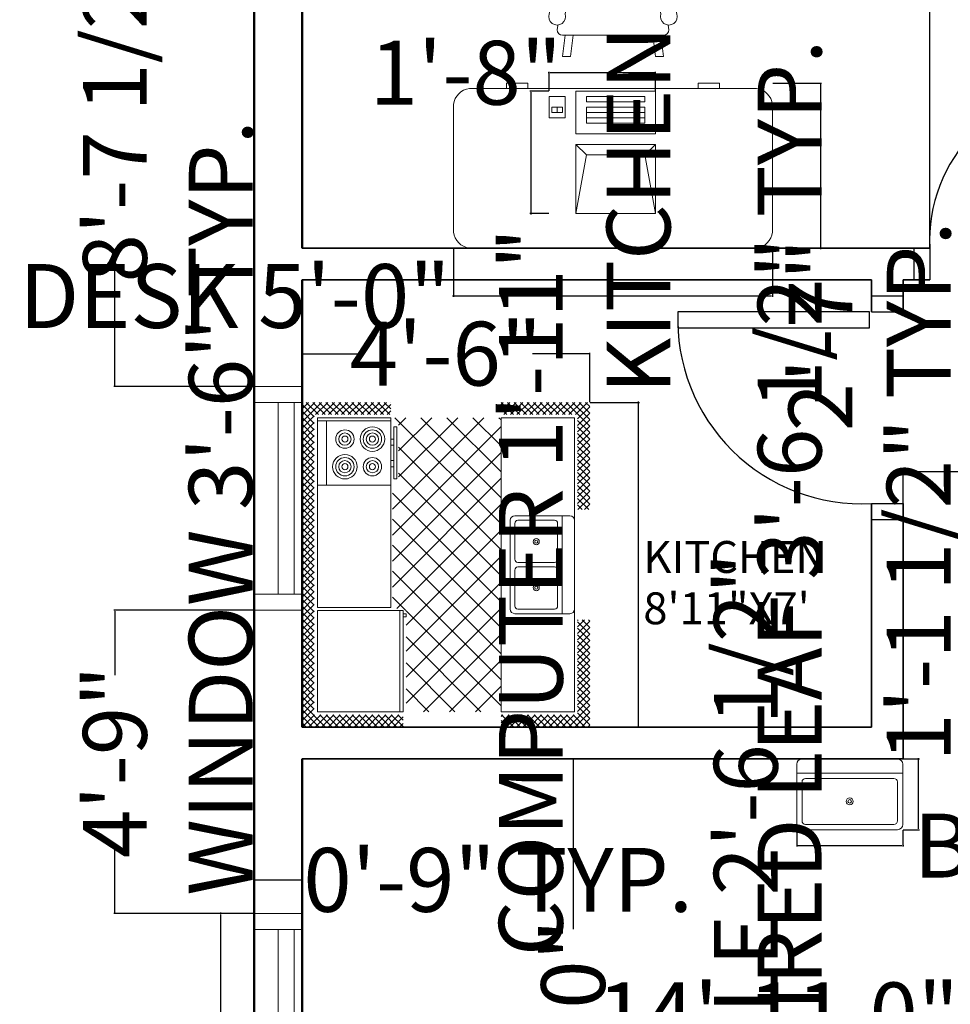
# Model space of a CAD drawing. Units: inches. Extents: x -52 to 472, y -40 to 644.
# Tile 3 of 6: x -21 to 154, y 164 to 349. Entities that reach past the tile are written whole.
import ezdxf

# ---------------------------------------------------------------- set-up
doc = ezdxf.new("R2010")
doc.units = ezdxf.units.IN
doc.header["$MEASUREMENT"] = 0
for name, color, linetype, lineweight in [('A-ANNO-DIMS', 7, 'Continuous', 13), ('A-ANNO-TEXT', 7, 'Continuous', 18), ('A-EQPM', 8, 'Continuous', 13), ('A-FLOR-FIXT', 8, 'Continuous', 13), ('DOORS', 2, 'Continuous', 25), ('FURNITURE', 6, 'Continuous', 13), ('INNER WALL', 1, 'Continuous', 35), ('OUTER WALL', 1, 'Continuous', 50), ('S-PLUM', 151, 'Continuous', 18), ('WINDOWS', 4, 'Continuous', 20)]:
    doc.layers.add(name, color=color, linetype=linetype, lineweight=lineweight)
doc.styles.get("Standard").update_dxf_attribs({"font": 'arial.ttf'})
doc.dimstyles.get("Standard").update_dxf_attribs({"dimtxt": 12, "dimasz": 0.18, "dimexe": 0.18, "dimexo": 0.0625, "dimgap": 0.09, "dimtad": 0, "dimdec": 1, "dimzin": 0, "dimdsep": 46, "dimlunit": 3, "dimtxsty": 'Standard', "dimcen": 0.09, "dimadec": 0, "dimazin": 0, "dimtfac": 1, "dimtdec": 1, "dimtofl": 0, "dimtmove": 0, "dimatfit": 3, "dimfxl": 1, "dimtolj": 1, "dimtzin": 0, "dimarcsym": 0})

# ---------------------------------------------------------------- blocks, each defined once
blk = doc.blocks.new('Chair - Rocking')
for p, q in [((-8, -4.5), (-10, -1.5)), ((8, -4.5), (10, -1.5)), ((-7.5, -4.5), (-7, -7)), ((-6.5, -7), (-7.02225, -4.43)), ((-4.5, -7), (-4.96674, -4.19951)), ((-4, -7), (-4.40532, -4.16272)), ((-1.5, -4.05012), (-1.5, -7)), ((-1, -7), (-1, -4.05012)), ((1, -7), (1, -4.04655)), ((1.5, -4.05012), (1.5, -7)), ((4, -7), (4.40187, -4.18694)), ((4.5, -7), (4.96761, -4.19437)), ((6.5, -7), (7, -4.4057)), ((7.5, -4.5), (7, -7)), ((-8.23428, -6.99939), (-8.3093, -7.47958)), ((-8.23041, -7), (8.23915, -7)), ((8.31071, -7.48854), (8.23449, -7.00073)), ((-9, -7.5), (-12, -18.49999)), ((-7, -7.5), (-9, -7.5)), ((-9, -18.49999), (-7, -7.5)), ((7, -7.5), (9, -7.5)), ((9, -18.49999), (7, -7.5)), ((9, -7.5), (12, -18.49999)), ((-10.36644, -20.64523), (-10.5, -21.49999)), ((10.5, -21.49999), (10.3575, -20.58798)), ((-9, -22.49999), (-9.5, -26.49999)), ((0, -22.49999), (-9.5, -22.49999)), ((-8, -26.49999), (-7.5, -22.49999)), ((0, -22.49999), (9.5, -22.49999)), ((8, -26.49999), (7.5, -22.49999)), ((9, -22.49999), (9.5, -26.49999)), ((-9.5, -26.49999), (-8, -26.49999)), ((9.5, -26.49999), (8, -26.49999))]:
    blk.add_line(p, q)
for centre, radius, start, end in [((0, -34.08333), 34.08333, 72.93847, 107.0615), ((0, -68.25004), 64.25, 93.92211, 97.15267), ((0, -68.25004), 64.25, 82.84733, 93.92211), ((-10.5, -18.99999), 1.58114, 161.5651, 18.43495), ((10.5, -18.99999), 1.58114, 161.5651, 18.43495), ((-9.5, -21.49999), 1, 180, 270), ((9.5, -21.49999), 1, 270, 0)]:
    blk.add_arc(centre, radius, start, end)
blk = doc.blocks.new('Computer Terminal')
for p, q in [((-10, 11.5), (5, 11.5)), ((-8, 0.5), (-10, 11.5)), ((-10, -1.5), (-10, 11.5)), ((5, 11.5), (3, 0.5)), ((5, 11.5), (5, -1.5)), ((-10, -1.5), (-8, 0.5)), ((3, 0.5), (-8, 0.5)), ((3, 0.5), (5, -1.5)), ((5, -1.5), (-10, -1.5)), ((-10, -11.5), (-10, -3.5)), ((-10, -3.5), (5, -3.5)), ((5, -3.5), (5, -11.5)), ((-8, -5.5), (-8, -8.5)), ((3, -5.5), (-8, -5.5)), ((3, -8.5), (3, -5.5)), ((3, -6.5), (-8, -6.5)), ((10, -6.5), (7, -6.5)), ((7, -6.5), (7, -10.5)), ((10, -10.5), (10, -6.5)), ((-8, -7.5), (3, -7.5)), ((-8, -8.5), (3, -8.5)), ((9.5, -7.5), (7.5, -7.5)), ((7.5, -7.5), (7.5, -8.5)), ((7.5, -8.5), (9.5, -8.5)), ((8.5, -7.5), (8.5, -8.5)), ((9.5, -8.5), (9.5, -7.5)), ((-8, -9.5), (-8, -10.5)), ((3, -9.5), (-8, -9.5)), ((-8, -10.5), (3, -10.5)), ((3, -10.5), (3, -9.5)), ((7, -10.5), (10, -10.5)), ((5, -11.5), (-10, -11.5))]:
    blk.add_line(p, q)
blk = doc.blocks.new('Desk - 30 x 60 in.')
for p, q in [((-26.999995, 0), (26.999995, 0)), ((-29.999995, -27), (-29.999995, -3)), ((29.999995, -3), (29.999995, -27)), ((26.999995, -30), (-26.999995, -30)), ((-20.000005, -30), (-20.000005, -31)), ((-20.000005, -31), (-16.000005, -31)), ((-16.000005, -31), (-16.000005, -30)), ((15.999995, -31), (15.999995, -30)), ((19.999995, -31), (15.999995, -31)), ((19.999995, -30), (19.999995, -31))]:
    blk.add_line(p, q)
for centre, start, end in [((-26.499995, -3.5), 98.1301, 171.8699), ((26.499995, -3.5), 8.130102, 81.8699), ((-26.499995, -26.5), 188.1301, 261.8699), ((26.499995, -26.5), 278.1301, 351.8699)]:
    blk.add_arc(centre, 3.535534, start, end)
blk = doc.blocks.new('Kitchen Layout - 7 x 8 ft')
for p, q in [((-5, 81.32), (2.68, 89)), ((-5, 83.44), (0.56, 89)), ((-5, 85.56), (-1.56, 89)), ((-5, 87.68), (-3.68, 89)), ((-1, 84.97), (-5, 88.97)), ((-1, 82.85), (-5, 86.85)), ((1.09, 85), (-2.91, 89)), ((3.21, 85), (-0.79, 89)), ((0.81, 85), (4.81, 89)), ((5.34, 85), (1.34, 89)), ((2.93, 85), (6.93, 89)), ((7.46, 85), (3.46, 89)), ((5.05, 85), (9.05, 89)), ((9.58, 85), (5.58, 89)), ((7.17, 85), (11.17, 89)), ((11.7, 85), (7.7, 89)), ((9.29, 85), (13.29, 89)), ((13.82, 85), (9.82, 89)), ((11.41, 85), (15.41, 89)), ((15.94, 85), (11.94, 89)), ((13.53, 85), (17.53, 89)), ((18.06, 85), (14.06, 89)), ((15.65, 85), (19.65, 89)), ((20.18, 85), (16.18, 89)), ((17.78, 85), (21.78, 89)), ((22.31, 85), (18.31, 89)), ((19.9, 85), (23.9, 89)), ((24.43, 85), (20.43, 89)), ((22.02, 85), (26.02, 89)), ((26.55, 85), (22.55, 89)), ((24.14, 85), (28.14, 89)), ((28.67, 85), (24.67, 89)), ((26.26, 85), (30.26, 89)), ((30.79, 85), (26.79, 89)), ((28.38, 85), (32.38, 89)), ((32.91, 85), (28.91, 89)), ((30.5, 85), (34.5, 89)), ((35.03, 85), (31.03, 89)), ((32.63, 85), (36.63, 89)), ((37.16, 85), (33.16, 89)), ((34.75, 85), (38.75, 89)), ((39.28, 85), (35.28, 89)), ((36.87, 85), (40.87, 89)), ((41.4, 85), (37.4, 89)), ((38.99, 85), (42.99, 89)), ((43.52, 85), (39.52, 89)), ((41.11, 85), (45.11, 89)), ((45.64, 85), (41.64, 89)), ((43.23, 85), (47.23, 89)), ((47.76, 85), (43.76, 89)), ((45.35, 85), (49.35, 89)), ((49.88, 85), (45.88, 89)), ((47.47, 85), (51.47, 89)), ((52, 85), (48, 89)), ((49.6, 85), (53.6, 89)), ((54.13, 85), (50.13, 89)), ((51.72, 85), (55.72, 89)), ((56.25, 85), (52.25, 89)), ((53.84, 85), (57.84, 89)), ((58.37, 85), (54.37, 89)), ((55.96, 85), (59.96, 89)), ((60.49, 85), (56.49, 89)), ((58.08, 85), (62.08, 89)), ((62.61, 85), (58.61, 89)), ((60.2, 85), (64.2, 89)), ((64.73, 85), (60.73, 89)), ((62.32, 85), (66.32, 89)), ((66.85, 85), (62.85, 89)), ((64.45, 85), (68.45, 89)), ((68.97, 85), (64.97, 89)), ((66.57, 85), (70.57, 89)), ((71.1, 85), (67.1, 89)), ((68.69, 85), (72.69, 89)), ((73.22, 85), (69.22, 89)), ((70.81, 85), (74.81, 89)), ((75.34, 85), (71.34, 89)), ((72.93, 85), (76.93, 89)), ((77.46, 85), (73.46, 89)), ((75.05, 85), (79.05, 89)), ((79.58, 85), (75.58, 89)), ((77.17, 85), (81.17, 89)), ((81.7, 85), (77.7, 89)), ((79.29, 85), (83.29, 89)), ((83.82, 85), (79.82, 89)), ((81.42, 85), (85.42, 89)), ((85.95, 85), (81.95, 89)), ((83.54, 85), (87.54, 89)), ((88.07, 85), (84.07, 89)), ((85.66, 85), (89.66, 89)), ((90.19, 85), (86.19, 89)), ((87.78, 85), (91.78, 89)), ((92.31, 85), (88.31, 89)), ((89.9, 85), (93.9, 89)), ((94.43, 85), (90.43, 89)), ((92.02, 85), (96.02, 89)), ((96.55, 85), (92.55, 89)), ((94.14, 85), (98.14, 89)), ((101, 82.67), (94.67, 89)), ((96.27, 85), (100.27, 89)), ((101, 84.79), (96.79, 89)), ((97, 83.61), (101, 87.61)), ((101, 86.92), (98.92, 89)), ((-1, 80.73), (-5, 84.73)), ((34, 84), (96, 84)), ((34, 60), (34, 84)), ((96, 84), (96, 60)), ((97, 81.49), (101, 85.49)), ((101, 80.55), (97, 84.55)), ((-5, 79.19), (-1, 83.19)), ((-1, 78.61), (-5, 82.61)), ((-5, 77.07), (-1, 81.07)), ((-1, 76.49), (-5, 80.49)), ((74, 81), (95, 81)), ((97, 79.37), (101, 83.37)), ((101, 78.43), (97, 82.43)), ((97, 77.25), (101, 81.25)), ((-5, 74.95), (-1, 78.95)), ((-1, 74.36), (-5, 78.36)), ((101, 76.31), (97, 80.31)), ((97, 75.13), (101, 79.13)), ((101, 74.19), (97, 78.19)), ((-5, 72.83), (-1, 76.83)), ((-1, 72.24), (-5, 76.24)), ((-5, 70.71), (-1, 74.71)), ((-1, 70.12), (-5, 74.12)), ((97, 73.01), (101, 77.01)), ((101, 72.07), (97, 76.07)), ((97, 70.89), (101, 74.89)), ((101, 69.95), (97, 73.95)), ((-5, 68.59), (-1, 72.59)), ((-1, 68), (-5, 72)), ((97, 68.76), (101, 72.76)), ((101, 67.82), (97, 71.82)), ((-5, 66.47), (-1, 70.47)), ((-1, 65.88), (-5, 69.88)), ((-5, 64.35), (-1, 68.35)), ((-1, 63.76), (-5, 67.76)), ((97, 66.64), (101, 70.64)), ((101, 65.7), (97, 69.7)), ((97, 64.52), (101, 68.52)), ((101, 63.58), (97, 67.58)), ((-5, 62.22), (-1, 66.22)), ((-1, 61.64), (-5, 65.64)), ((97, 62.4), (101, 66.4)), ((101, 61.46), (97, 65.46)), ((-5, 60.1), (-1, 64.1)), ((-1, 59.52), (-5, 63.52)), ((-5, 57.98), (-1, 61.98)), ((-1, 57.39), (-5, 61.39)), ((97, 60.28), (101, 64.28)), ((100.34, 60), (97, 63.34)), ((98.22, 60), (97, 61.22)), ((98.84, 60), (101, 62.16)), ((-1.73, 56), (-5, 59.27)), ((-4.86, 56), (-1, 59.86)), ((10.4, 24), (45.9, 59.5)), ((18.88, 24), (54.38, 59.5)), ((27.37, 24), (62.87, 59.5)), ((33.03, 55.11), (37.41, 59.5)), ((67.71, 24), (33.68, 58.04)), ((96, 60), (34, 60)), ((35.85, 24), (71.35, 59.5)), ((76.2, 24), (40.7, 59.5)), ((84.68, 24), (49.18, 59.5)), ((93.17, 24), (57.67, 59.5)), ((61.31, 24), (96, 58.69)), ((96, 29.65), (66.15, 59.5)), ((80, 60), (80, 59)), ((82, 59), (82, 60)), ((87, 59), (87, 60)), ((89, 60), (89, 59)), ((100.96, 60), (101, 60.04)), ((-3.85, 56), (-5, 57.15)), ((-2.74, 56), (-1, 57.74)), ((0, 57), (33, 57)), ((0, 30.57), (24.43, 55)), ((0, 39.06), (15.94, 55)), ((0, 47.54), (7.46, 55)), ((1.91, 24), (32.91, 55)), ((33.77, 24), (2.77, 55)), ((42.26, 24), (11.26, 55)), ((50.74, 24), (19.74, 55)), ((59.23, 24), (28.23, 55)), ((31, 55), (31, 56)), ((32, 55), (31, 55)), ((32, 56), (32, 55)), ((44.34, 24), (77.84, 57.5)), ((52.82, 24), (86.32, 57.5)), ((96, 38.14), (76.64, 57.5)), ((96, 46.63), (85.13, 57.5)), ((96, 55.11), (93.57, 57.54)), ((25.29, 24), (0, 49.29)), ((69.79, 24), (96, 50.21)), ((16.8, 24), (0, 40.8)), ((78.28, 24), (96, 41.72)), ((8.32, 24), (0, 32.32)), ((86.76, 24), (96, 33.24)), ((-5, 21.92), (-2.92, 24)), ((-5, 19.8), (-1, 23.8)), ((-1, 19.21), (-5, 23.21)), ((-1, 21.33), (-3.67, 24)), ((-1, 23.45), (-1.55, 24)), ((0, 24), (96, 24)), ((0, 0), (0, 24)), ((95.25, 24), (96, 24.75)), ((96, 24), (96, 0)), ((97, 22.1), (98.9, 24)), ((97, 19.97), (101, 23.97)), ((101, 19.03), (97, 23.03)), ((101, 21.16), (98.16, 24)), ((101, 23.28), (100.28, 24)), ((-5, 17.68), (-1, 21.68)), ((-1, 17.09), (-5, 21.09)), ((-5, 15.55), (-1, 19.55)), ((97, 17.85), (101, 21.85)), ((101, 16.91), (97, 20.91)), ((97, 15.73), (101, 19.73)), ((-1, 14.97), (-5, 18.97)), ((-5, 13.43), (-1, 17.43)), ((-1, 12.85), (-5, 16.85)), ((47.25, 6.5), (47.25, 18.5)), ((48.75, 18.5), (48.75, 6.5)), ((101, 14.79), (97, 18.79)), ((97, 13.61), (101, 17.61)), ((101, 12.67), (97, 16.67)), ((-5, 11.31), (-1, 15.31)), ((-1, 10.73), (-5, 14.73)), ((-5, 9.19), (-1, 13.19)), ((97, 11.49), (101, 15.49)), ((101, 10.55), (97, 14.55)), ((97, 9.37), (101, 13.37)), ((-1, 8.6), (-5, 12.6)), ((-5, 7.07), (-1, 11.07)), ((-1, 6.48), (-5, 10.48)), ((101, 8.43), (97, 12.43)), ((97, 7.25), (101, 11.25)), ((101, 6.31), (97, 10.31)), ((-5, 4.95), (-1, 8.95)), ((-1, 4.36), (-5, 8.36)), ((-5, 2.83), (-1, 6.83)), ((97, 5.12), (101, 9.12)), ((101, 4.18), (97, 8.18)), ((97, 3), (101, 7)), ((-1, 2.24), (-5, 6.24)), ((-5, 0.71), (-1, 4.71)), ((-1, 0.12), (-5, 4.12)), ((64, 4), (32, 4)), ((101, 2.06), (97, 6.06)), ((97, 0.88), (101, 4.88)), ((101, -0.06), (97, 3.94)), ((-5, -1.42), (-1, 2.58)), ((2, -5), (-5, 2)), ((-5, -3.54), (-1, 0.46)), ((96, 0), (0, 0)), ((93.24, -5), (101, 2.76)), ((95.36, -5), (101, 0.64)), ((101, -2.18), (97, 1.82)), ((-0.12, -5), (-5, -0.12)), ((-2.25, -5), (-5, -2.25)), ((-4.34, -5), (-0.34, -1)), ((-2.22, -5), (1.78, -1)), ((-0.1, -5), (3.9, -1)), ((4.12, -5), (0.12, -1)), ((2.02, -5), (6.02, -1)), ((6.24, -5), (2.24, -1)), ((4.14, -5), (8.14, -1)), ((8.36, -5), (4.36, -1)), ((6.27, -5), (10.27, -1)), ((10.48, -5), (6.48, -1)), ((8.39, -5), (12.39, -1)), ((12.6, -5), (8.6, -1)), ((10.51, -5), (14.51, -1)), ((14.73, -5), (10.73, -1)), ((12.63, -5), (16.63, -1)), ((16.85, -5), (12.85, -1)), ((14.75, -5), (18.75, -1)), ((18.97, -5), (14.97, -1)), ((16.87, -5), (20.87, -1)), ((21.09, -5), (17.09, -1)), ((18.99, -5), (22.99, -1)), ((23.21, -5), (19.21, -1)), ((21.11, -5), (25.11, -1)), ((25.33, -5), (21.33, -1)), ((23.24, -5), (27.24, -1)), ((27.45, -5), (23.45, -1)), ((25.36, -5), (29.36, -1)), ((29.57, -5), (25.57, -1)), ((27.48, -5), (30, -2.48)), ((30, -3.3), (27.7, -1)), ((30, -1.18), (29.82, -1)), ((66, -2.54), (67.54, -1)), ((66, -4.66), (69.66, -1)), ((69.88, -5), (66, -1.12)), ((67.78, -5), (71.78, -1)), ((72, -5), (68, -1)), ((69.9, -5), (73.9, -1)), ((74.12, -5), (70.12, -1)), ((72.03, -5), (76.03, -1)), ((76.24, -5), (72.24, -1)), ((74.15, -5), (78.15, -1)), ((78.36, -5), (74.36, -1)), ((76.27, -5), (80.27, -1)), ((80.49, -5), (76.49, -1)), ((78.39, -5), (82.39, -1)), ((82.61, -5), (78.61, -1)), ((80.51, -5), (84.51, -1)), ((84.73, -5), (80.73, -1)), ((82.63, -5), (86.63, -1)), ((86.85, -5), (82.85, -1)), ((84.75, -5), (88.75, -1)), ((88.97, -5), (84.97, -1)), ((86.88, -5), (90.88, -1)), ((91.09, -5), (87.09, -1)), ((89, -5), (93, -1)), ((93.21, -5), (89.21, -1)), ((91.12, -5), (95.12, -1)), ((95.34, -5), (91.34, -1)), ((97.46, -5), (93.46, -1)), ((99.58, -5), (95.58, -1)), ((101, -4.3), (97, -0.3)), ((97.48, -5), (101, -1.48)), ((-4.37, -5), (-5, -4.37)), ((29.6, -5), (30, -4.6)), ((67.76, -5), (66, -3.24)), ((99.6, -5), (101, -3.6))]:
    blk.add_line(p, q)
for points in [[(0, 56), (0, 84), (33, 84), (33, 56)], [(74, 60), (74, 84), (95, 84), (95, 60)], [(76, 58), (76, 59), (93, 59), (93, 58)]]:
    blk.add_lwpolyline(points, close=True)
for points in [[(32, 1.5), (32, 19.5)], [(33.5, 21), (62.5, 21)], [(34.5, 19.5), (46.25, 19.5)], [(49.75, 19.5), (61.5, 19.5)], [(64, 19.5), (64, 1.5)], [(33.5, 6.5), (33.5, 18.5)], [(62.5, 18.5), (62.5, 6.5)], [(46.25, 5.5), (34.5, 5.5)], [(61.5, 5.5), (49.75, 5.5)], [(62.5, 0), (33.5, 0)]]:
    blk.add_lwpolyline(points)
for centre, radius in [((80, 75), 4), ((80, 75), 3), ((89, 75), 3), ((80, 75), 2), ((80, 75), 1), ((89, 75), 2), ((89, 75), 1), ((80, 66), 3), ((80, 66), 2), ((89, 66), 4), ((89, 66), 3), ((89, 66), 2), ((80, 66), 1), ((89, 66), 1), ((40.5, 12.5), 1), ((40.5, 12.5), 0.5), ((55.5, 12.5), 1), ((55.5, 12.5), 0.5)]:
    blk.add_circle(centre, radius)
for centre, radius, start, end in [((33.5, 19.5), 1.5, 90, 180), ((34.5, 18.5), 1, 90, 180), ((46.25, 18.5), 1, 0, 90), ((49.75, 18.5), 1, 90, 180), ((61.5, 18.5), 1, 0, 90), ((62.5, 19.5), 1.5, 0, 90), ((34.5, 6.5), 1, 180, 270), ((46.25, 6.5), 1, 270, 0), ((49.75, 6.5), 1, 180, 270), ((61.5, 6.5), 1, 270, 0), ((33.5, 1.5), 1.5, 180, 270), ((62.5, 1.5), 1.5, 270, 0)]:
    blk.add_arc(centre, radius, start, end)
blk = doc.blocks.new('Sink-single - 30 in top')
blk.add_line((-15, -3.999996), (15, -3.999996))
for points in [[(-13.5, 0), (13.5, 0)], [(-15, -18.499996), (-15, -1.5)], [(15, -1.5), (15, -18.499996)], [(-12.5, -5.499996), (12.5, -5.499996)], [(-13.5, -17.499996), (-13.5, -6.499996)], [(13.5, -6.499996), (13.5, -17.499996)], [(12.5, -18.499996), (-12.5, -18.499996)], [(13.5, -19.999996), (-13.5, -19.999996)]]:
    blk.add_lwpolyline(points)
for radius in [1, 0.5]:
    blk.add_circle((0, -11.999996), radius)
for centre, radius, start, end in [((-13.5, -1.5), 1.5, 90, 180), ((13.5, -1.5), 1.5, 0, 90), ((-12.5, -6.499996), 1, 90, 180), ((12.5, -6.499996), 1, 0, 90), ((-13.5, -18.499996), 1.5, 180, 270), ((-12.5, -17.499996), 1, 180, 270), ((12.5, -17.499996), 1, 270, 0), ((13.5, -18.499996), 1.5, 270, 0)]:
    blk.add_arc(centre, radius, start, end)
blk = doc.blocks.new('*D15')
at = {"layer": 'A-ANNO-DIMS', "color": 0, "lineweight": -2, "transparency": 16777216}
for p, q in [((145.13, 258.39), (145.13, 264.49)), ((145.31, 264.31), (174.59, 264.31)), ((249.95, 264.31), (220.67, 264.31)), ((250.13, 261.39), (250.13, 264.49))]:
    blk.add_line(p, q, dxfattribs=at)
at = {"layer": 'A-ANNO-DIMS', "color": 0, "transparency": 16777216}
for points in [[(145.31, 264.34), (145.31, 264.28), (145.13, 264.31)], [(249.95, 264.34), (249.95, 264.28), (250.13, 264.31)]]:
    blk.add_solid(points, dxfattribs=at)
at = {"layer": 'Defpoints', "color": 0, "transparency": 16777216}
for p in [(250.13, 264.31), (250.13, 261.33), (145.13, 258.33)]:
    blk.add_point(p, dxfattribs=at)
at = {"layer": 'A-ANNO-DIMS', "color": 0, "transparency": 16777216, "insert": (197.63, 264.31), "char_height": 12, "attachment_point": 5}
blk.add_mtext('\\A1;8\'-9.0"', dxfattribs=at)
blk = doc.blocks.new('*D16')
at = {"layer": 'A-ANNO-DIMS', "color": 0, "lineweight": -2, "transparency": 16777216}
for p, q in [((88.57, 210.33), (82.89, 210.33)), ((83.07, 210.15), (83.07, 178.36)), ((83.07, 100.51), (83.07, 132.3)), ((88.57, 100.33), (82.89, 100.33))]:
    blk.add_line(p, q, dxfattribs=at)
at = {"layer": 'A-ANNO-DIMS', "color": 0, "transparency": 16777216}
for points in [[(83.04, 210.15), (83.1, 210.15), (83.07, 210.33)], [(83.04, 100.51), (83.1, 100.51), (83.07, 100.33)]]:
    blk.add_solid(points, dxfattribs=at)
at = {"layer": 'Defpoints', "color": 0, "transparency": 16777216}
for p in [(88.63, 210.33), (83.07, 100.33), (88.63, 100.33)]:
    blk.add_point(p, dxfattribs=at)
at = {"layer": 'A-ANNO-DIMS', "color": 0, "transparency": 16777216, "insert": (83.07, 155.33), "char_height": 12, "attachment_point": 5, "rotation": 90}
blk.add_mtext('\\A1;9\'-2.0"', dxfattribs=at)
blk = doc.blocks.new('*D17')
at = {"layer": 'A-ANNO-DIMS', "color": 0, "lineweight": -2, "transparency": 16777216}
for p, q in [((32.13, 162.39), (32.13, 162.51)), ((32.31, 162.33), (89.84, 162.33)), ((210.95, 162.33), (153.42, 162.33)), ((211.13, 162.39), (211.13, 162.51))]:
    blk.add_line(p, q, dxfattribs=at)
at = {"layer": 'A-ANNO-DIMS', "color": 0, "transparency": 16777216}
for points in [[(32.31, 162.36), (32.31, 162.3), (32.13, 162.33)], [(210.95, 162.36), (210.95, 162.3), (211.13, 162.33)]]:
    blk.add_solid(points, dxfattribs=at)
at = {"layer": 'Defpoints', "color": 0, "transparency": 16777216}
for p in [(32.13, 162.33), (32.13, 162.33), (211.13, 162.33)]:
    blk.add_point(p, dxfattribs=at)
at = {"layer": 'A-ANNO-DIMS', "color": 0, "transparency": 16777216, "insert": (121.63, 162.33), "char_height": 12, "attachment_point": 5}
blk.add_mtext('\\A1;14\'-11.0"', dxfattribs=at)
blk = doc.blocks.new('WIN-36IN')
for p, q in [((9, 42), (0, 42)), ((9, 39), (0, 39)), ((4.5, 3), (4.5, 39)), ((7.5, 3), (7.5, 39)), ((0, 3), (9, 3)), ((0, 0), (9, 0))]:
    blk.add_line(p, q)
blk = doc.blocks.new('*D26')
at = {"layer": 'A-ANNO-DIMS', "color": 0, "lineweight": -2, "transparency": 16777216}
for p, q in [((23.07, 181.31), (16.65, 181.31)), ((16.83, 181.31), (16.83, 181.49)), ((16.83, 139.49), (16.83, 181.13)), ((23.07, 139.31), (16.65, 139.31))]:
    blk.add_line(p, q, dxfattribs=at)
at = {"layer": 'A-ANNO-DIMS', "color": 0, "transparency": 16777216}
for points in [[(16.8, 181.13), (16.86, 181.13), (16.83, 181.31)], [(16.8, 139.49), (16.86, 139.49), (16.83, 139.31)]]:
    blk.add_solid(points, dxfattribs=at)
at = {"layer": 'Defpoints', "color": 0, "transparency": 16777216}
for p in [(16.83, 181.31), (23.13, 181.31), (23.13, 139.31)]:
    blk.add_point(p, dxfattribs=at)
at = {"layer": 'A-ANNO-DIMS', "color": 0, "transparency": 16777216, "insert": (16.83, 257.5), "char_height": 12, "attachment_point": 5, "rotation": 90}
blk.add_mtext('\\A1;WINDOW 3\'-6" TYP.', dxfattribs=at)
blk = doc.blocks.new('*D27')
at = {"layer": 'A-ANNO-DIMS', "color": 0, "lineweight": -2, "transparency": 16777216}
for p, q in [((23.13, 181.37), (23.13, 187.79)), ((23.31, 187.61), (31.95, 187.61)), ((32.13, 181.37), (32.13, 187.79)), ((32.13, 187.61), (32.31, 187.61))]:
    blk.add_line(p, q, dxfattribs=at)
at = {"layer": 'A-ANNO-DIMS', "color": 0, "transparency": 16777216}
for points in [[(23.31, 187.64), (23.31, 187.58), (23.13, 187.61)], [(31.95, 187.64), (31.95, 187.58), (32.13, 187.61)]]:
    blk.add_solid(points, dxfattribs=at)
at = {"layer": 'Defpoints', "color": 0, "transparency": 16777216}
for p in [(32.13, 187.61), (23.13, 181.31), (32.13, 181.31)]:
    blk.add_point(p, dxfattribs=at)
at = {"layer": 'A-ANNO-DIMS', "color": 0, "transparency": 16777216, "insert": (68.98, 187.61), "char_height": 12, "attachment_point": 5}
blk.add_mtext('\\A1;0\'-9" TYP.', dxfattribs=at)
blk = doc.blocks.new('*D32')
at = {"layer": 'A-ANNO-DIMS', "color": 0, "lineweight": -2, "transparency": 16777216}
for p, q in [((125.1, 196.98), (125.1, 193.87)), ((145.03, 196.98), (145.03, 193.87)), ((125.28, 194.05), (144.85, 194.05)), ((145.03, 194.05), (145.21, 194.05))]:
    blk.add_line(p, q, dxfattribs=at)
at = {"layer": 'A-ANNO-DIMS', "color": 0, "transparency": 16777216}
for points in [[(125.28, 194.08), (125.28, 194.02), (125.1, 194.05)], [(144.85, 194.08), (144.85, 194.02), (145.03, 194.05)]]:
    blk.add_solid(points, dxfattribs=at)
at = {"layer": 'Defpoints', "color": 0, "transparency": 16777216}
for p in [(125.1, 197.04), (145.03, 197.04), (145.03, 194.05)]:
    blk.add_point(p, dxfattribs=at)
at = {"layer": 'A-ANNO-DIMS', "color": 0, "transparency": 16777216, "insert": (209.09, 194.05), "char_height": 12, "attachment_point": 5}
blk.add_mtext('\\A1;BASIN 1\'-8" TYP.', dxfattribs=at)
blk = doc.blocks.new('*D33')
at = {"layer": 'A-ANNO-DIMS', "color": 0, "lineweight": -2, "transparency": 16777216}
for p, q in [((145.09, 210.33), (148.2, 210.33)), ((148.02, 210.33), (148.02, 210.51)), ((148.02, 197.22), (148.02, 210.15)), ((145.09, 197.04), (148.2, 197.04))]:
    blk.add_line(p, q, dxfattribs=at)
at = {"layer": 'A-ANNO-DIMS', "color": 0, "transparency": 16777216}
for points in [[(147.99, 210.15), (148.05, 210.15), (148.02, 210.33)], [(147.99, 197.22), (148.05, 197.22), (148.02, 197.04)]]:
    blk.add_solid(points, dxfattribs=at)
at = {"layer": 'Defpoints', "color": 0, "transparency": 16777216}
for p in [(145.03, 210.33), (148.02, 210.33), (145.03, 197.04)]:
    blk.add_point(p, dxfattribs=at)
at = {"layer": 'A-ANNO-DIMS', "color": 0, "transparency": 16777216, "insert": (148.02, 260.59), "char_height": 12, "attachment_point": 5, "rotation": 90}
blk.add_mtext('\\A1;1\'-1 1/2" TYP.', dxfattribs=at)
blk = doc.blocks.new('*D38')
at = {"layer": 'A-ANNO-DIMS', "color": 0, "lineweight": -2, "transparency": 16777216}
for p, q in [((78.5, 335.81), (74.94, 335.81)), ((75.12, 335.63), (75.12, 312.99)), ((78.5, 312.81), (74.94, 312.81)), ((75.12, 312.81), (75.12, 312.63))]:
    blk.add_line(p, q, dxfattribs=at)
at = {"layer": 'A-ANNO-DIMS', "color": 0, "transparency": 16777216}
for points in [[(75.09, 335.63), (75.15, 335.63), (75.12, 335.81)], [(75.09, 312.99), (75.15, 312.99), (75.12, 312.81)]]:
    blk.add_solid(points, dxfattribs=at)
at = {"layer": 'Defpoints', "color": 0, "transparency": 16777216}
for p in [(78.57, 335.81), (75.12, 312.81), (78.57, 312.81)]:
    blk.add_point(p, dxfattribs=at)
at = {"layer": 'A-ANNO-DIMS', "color": 0, "transparency": 16777216, "insert": (75.12, 241.71), "char_height": 12, "attachment_point": 5, "rotation": 90}
blk.add_mtext('\\A1;COMPUTER 1\'-11"', dxfattribs=at)
blk = doc.blocks.new('*D39')
at = {"layer": 'A-ANNO-DIMS', "color": 0, "lineweight": -2, "transparency": 16777216}
for p, q in [((78.57, 339.26), (78.39, 339.26)), ((78.57, 335.87), (78.57, 339.44)), ((98.39, 339.26), (78.75, 339.26)), ((98.57, 335.87), (98.57, 339.44))]:
    blk.add_line(p, q, dxfattribs=at)
at = {"layer": 'A-ANNO-DIMS', "color": 0, "transparency": 16777216}
for points in [[(78.75, 339.29), (78.75, 339.23), (78.57, 339.26)], [(98.39, 339.29), (98.39, 339.23), (98.57, 339.26)]]:
    blk.add_solid(points, dxfattribs=at)
at = {"layer": 'Defpoints', "color": 0, "transparency": 16777216}
for p in [(78.57, 339.26), (78.57, 335.81), (98.57, 335.81)]:
    blk.add_point(p, dxfattribs=at)
at = {"layer": 'A-ANNO-DIMS', "color": 0, "transparency": 16777216, "insert": (62.91, 339.26), "char_height": 12, "attachment_point": 5}
blk.add_mtext('\\A1;1\'-8"', dxfattribs=at)
blk = doc.blocks.new('*D42')
at = {"layer": 'A-ANNO-DIMS', "color": 0, "lineweight": -2, "transparency": 16777216}
for p, q in [((60.57, 306.25), (60.57, 297.13)), ((120.57, 306.25), (120.57, 297.13)), ((60.57, 297.31), (60.39, 297.31)), ((120.39, 297.31), (60.75, 297.31))]:
    blk.add_line(p, q, dxfattribs=at)
at = {"layer": 'A-ANNO-DIMS', "color": 0, "transparency": 16777216}
for points in [[(60.75, 297.34), (60.75, 297.28), (60.57, 297.31)], [(120.39, 297.34), (120.39, 297.28), (120.57, 297.31)]]:
    blk.add_solid(points, dxfattribs=at)
at = {"layer": 'Defpoints', "color": 0, "transparency": 16777216}
for p in [(60.57, 306.31), (120.57, 306.31), (60.57, 297.31)]:
    blk.add_point(p, dxfattribs=at)
at = {"layer": 'A-ANNO-DIMS', "color": 0, "transparency": 16777216, "insert": (19.49, 297.31), "char_height": 12, "attachment_point": 5}
blk.add_mtext('\\A1;DESK 5\'-0"', dxfattribs=at)
blk = doc.blocks.new('*D43')
at = {"layer": 'A-ANNO-DIMS', "color": 0, "lineweight": -2, "transparency": 16777216}
for p, q in [((120.63, 337.31), (129.75, 337.31)), ((129.57, 337.13), (129.57, 306.49)), ((120.63, 306.31), (129.75, 306.31)), ((129.57, 306.31), (129.57, 306.13))]:
    blk.add_line(p, q, dxfattribs=at)
at = {"layer": 'A-ANNO-DIMS', "color": 0, "transparency": 16777216}
for points in [[(129.54, 337.13), (129.6, 337.13), (129.57, 337.31)], [(129.54, 306.49), (129.6, 306.49), (129.57, 306.31)]]:
    blk.add_solid(points, dxfattribs=at)
at = {"layer": 'Defpoints', "color": 0, "transparency": 16777216}
for p in [(120.57, 337.31), (120.57, 306.31), (129.57, 306.31)]:
    blk.add_point(p, dxfattribs=at)
at = {"layer": 'A-ANNO-DIMS', "color": 0, "transparency": 16777216, "insert": (129.57, 289.99), "char_height": 12, "attachment_point": 5, "rotation": 90}
blk.add_mtext('\\A1;2\'-7"', dxfattribs=at)
blk = doc.blocks.new('*D52')
at = {"layer": 'A-ANNO-DIMS', "color": 0, "lineweight": -2, "transparency": 16777216}
for p, q in [((123.77, 136.75), (123.77, 136.93)), ((130.07, 136.75), (123.59, 136.75)), ((123.77, 94.51), (123.77, 136.57)), ((130.07, 94.33), (123.59, 94.33))]:
    blk.add_line(p, q, dxfattribs=at)
at = {"layer": 'A-ANNO-DIMS', "color": 0, "transparency": 16777216}
for points in [[(123.74, 136.57), (123.8, 136.57), (123.77, 136.75)], [(123.74, 94.51), (123.8, 94.51), (123.77, 94.33)]]:
    blk.add_solid(points, dxfattribs=at)
at = {"layer": 'Defpoints', "color": 0, "transparency": 16777216}
for p in [(123.77, 136.75), (130.13, 136.75), (130.13, 94.33)]:
    blk.add_point(p, dxfattribs=at)
at = {"layer": 'A-ANNO-DIMS', "color": 0, "transparency": 16777216, "insert": (123.77, 244.1), "char_height": 12, "attachment_point": 5, "rotation": 90}
blk.add_mtext('\\A1;PAIRED LEAF 3\'-6 1/2" TYP.', dxfattribs=at)
blk = doc.blocks.new('*D53')
at = {"layer": 'A-ANNO-DIMS', "color": 0, "lineweight": -2, "transparency": 16777216}
for p, q in [((130.13, 136.81), (130.13, 143.29)), ((130.31, 143.11), (169.37, 143.11)), ((169.55, 136.81), (169.55, 143.29)), ((169.55, 143.11), (169.73, 143.11))]:
    blk.add_line(p, q, dxfattribs=at)
at = {"layer": 'A-ANNO-DIMS', "color": 0, "transparency": 16777216}
for points in [[(130.31, 143.14), (130.31, 143.08), (130.13, 143.11)], [(169.37, 143.14), (169.37, 143.08), (169.55, 143.11)]]:
    blk.add_solid(points, dxfattribs=at)
at = {"layer": 'Defpoints', "color": 0, "transparency": 16777216}
for p in [(169.55, 143.11), (130.13, 136.75), (169.55, 136.75)]:
    blk.add_point(p, dxfattribs=at)
at = {"layer": 'A-ANNO-DIMS', "color": 0, "transparency": 16777216, "insert": (220.37, 143.11), "char_height": 12, "attachment_point": 5}
blk.add_mtext('\\A1;3\'-3 1/2" TYP.', dxfattribs=at)
blk = doc.blocks.new('*D60')
at = {"layer": 'A-ANNO-DIMS', "color": 0, "lineweight": -2, "transparency": 16777216}
for p, q in [((120.04, 63.4), (115.35, 63.4)), ((115.53, 63.4), (115.53, 63.58)), ((115.53, 33.11), (115.53, 63.22)), ((120.04, 32.93), (115.35, 32.93))]:
    blk.add_line(p, q, dxfattribs=at)
at = {"layer": 'A-ANNO-DIMS', "color": 0, "transparency": 16777216}
for points in [[(115.5, 63.22), (115.56, 63.22), (115.53, 63.4)], [(115.5, 33.11), (115.56, 33.11), (115.53, 32.93)]]:
    blk.add_solid(points, dxfattribs=at)
at = {"layer": 'Defpoints', "color": 0, "transparency": 16777216}
for p in [(115.53, 63.4), (120.1, 63.4), (120.1, 32.93)]:
    blk.add_point(p, dxfattribs=at)
at = {"layer": 'A-ANNO-DIMS', "color": 0, "transparency": 16777216, "insert": (115.53, 158.74), "char_height": 12, "attachment_point": 5, "rotation": 90}
blk.add_mtext('\\A1;COFFEE TABLE 2\'-6 1/2"', dxfattribs=at)
blk = doc.blocks.new('*D62')
at = {"layer": 'A-ANNO-DIMS', "color": 0, "lineweight": -2, "transparency": 16777216}
for p, q in [((95.36, 277.33), (95.36, 277.51)), ((86.27, 277.33), (95.54, 277.33)), ((95.36, 216.51), (95.36, 277.15)), ((86.27, 216.33), (95.54, 216.33))]:
    blk.add_line(p, q, dxfattribs=at)
at = {"layer": 'A-ANNO-DIMS', "color": 0, "transparency": 16777216}
for points in [[(95.33, 277.15), (95.39, 277.15), (95.36, 277.33)], [(95.33, 216.51), (95.39, 216.51), (95.36, 216.33)]]:
    blk.add_solid(points, dxfattribs=at)
at = {"layer": 'Defpoints', "color": 0, "transparency": 16777216}
for p in [(86.21, 277.33), (95.36, 277.33), (86.21, 216.33)]:
    blk.add_point(p, dxfattribs=at)
at = {"layer": 'A-ANNO-DIMS', "color": 0, "transparency": 16777216, "insert": (95.36, 354.29), "char_height": 12, "attachment_point": 5, "rotation": 90}
blk.add_mtext('\\A1;KITCHEN UNIT 5\'-1"', dxfattribs=at)
blk = doc.blocks.new('*D63')
at = {"layer": 'A-ANNO-DIMS', "color": 0, "lineweight": -2, "transparency": 16777216}
for p, q in [((32.12, 277.39), (32.12, 286.66)), ((32.3, 286.48), (42.88, 286.48)), ((86.03, 286.48), (75.44, 286.48)), ((86.21, 277.39), (86.21, 286.66))]:
    blk.add_line(p, q, dxfattribs=at)
at = {"layer": 'A-ANNO-DIMS', "color": 0, "transparency": 16777216}
for points in [[(32.3, 286.51), (32.3, 286.45), (32.12, 286.48)], [(86.03, 286.51), (86.03, 286.45), (86.21, 286.48)]]:
    blk.add_solid(points, dxfattribs=at)
at = {"layer": 'Defpoints', "color": 0, "transparency": 16777216}
for p in [(32.12, 286.48), (32.12, 277.33), (86.21, 277.33)]:
    blk.add_point(p, dxfattribs=at)
at = {"layer": 'A-ANNO-DIMS', "color": 0, "transparency": 16777216, "insert": (59.16, 286.48), "char_height": 12, "attachment_point": 5}
blk.add_mtext('\\A1;4\'-6"', dxfattribs=at)
blk = doc.blocks.new('*D67')
at = {"layer": 'A-ANNO-DIMS', "color": 0, "lineweight": -2, "transparency": 16777216}
for p, q in [((23.07, 383.81), (-3.25, 383.81)), ((-3.07, 383.63), (-3.07, 362.09)), ((-3.07, 280.49), (-3.07, 302.03)), ((23.07, 280.31), (-3.25, 280.31))]:
    blk.add_line(p, q, dxfattribs=at)
at = {"layer": 'A-ANNO-DIMS', "color": 0, "transparency": 16777216}
for points in [[(-3.1, 383.63), (-3.04, 383.63), (-3.07, 383.81)], [(-3.1, 280.49), (-3.04, 280.49), (-3.07, 280.31)]]:
    blk.add_solid(points, dxfattribs=at)
at = {"layer": 'Defpoints', "color": 0, "transparency": 16777216}
for p in [(23.13, 383.81), (-3.07, 280.31), (23.13, 280.31)]:
    blk.add_point(p, dxfattribs=at)
at = {"layer": 'A-ANNO-DIMS', "color": 0, "transparency": 16777216, "insert": (-3.07, 332.06), "char_height": 12, "attachment_point": 5, "rotation": 90}
blk.add_mtext('\\A1;8\'-7 1/2"', dxfattribs=at)
blk = doc.blocks.new('*D68')
at = {"layer": 'A-ANNO-DIMS', "color": 0, "lineweight": -2, "transparency": 16777216}
for p, q in [((23.07, 238.31), (-3.25, 238.31)), ((-3.07, 238.13), (-3.07, 226.09)), ((-3.07, 181.49), (-3.07, 193.53)), ((23.07, 181.31), (-3.25, 181.31))]:
    blk.add_line(p, q, dxfattribs=at)
at = {"layer": 'A-ANNO-DIMS', "color": 0, "transparency": 16777216}
for points in [[(-3.1, 238.13), (-3.04, 238.13), (-3.07, 238.31)], [(-3.1, 181.49), (-3.04, 181.49), (-3.07, 181.31)]]:
    blk.add_solid(points, dxfattribs=at)
at = {"layer": 'Defpoints', "color": 0, "transparency": 16777216}
for p in [(23.13, 238.31), (-3.07, 181.31), (23.13, 181.31)]:
    blk.add_point(p, dxfattribs=at)
at = {"layer": 'A-ANNO-DIMS', "color": 0, "transparency": 16777216, "insert": (-3.07, 209.81), "char_height": 12, "attachment_point": 5, "rotation": 90}
blk.add_mtext('\\A1;4\'-9"', dxfattribs=at)
blk = doc.blocks.new('*D80')
at = {"layer": 'A-ANNO-DIMS', "color": 0, "lineweight": -2, "transparency": 16777216}
for p, q in [((150.13, 306.39), (150.13, 508.71)), ((150.31, 508.53), (179.95, 508.53)), ((180.13, 306.39), (180.13, 508.71)), ((180.13, 508.53), (180.31, 508.53))]:
    blk.add_line(p, q, dxfattribs=at)
at = {"layer": 'A-ANNO-DIMS', "color": 0, "transparency": 16777216}
for points in [[(150.31, 508.56), (150.31, 508.5), (150.13, 508.53)], [(179.95, 508.56), (179.95, 508.5), (180.13, 508.53)]]:
    blk.add_solid(points, dxfattribs=at)
at = {"layer": 'Defpoints', "color": 0, "transparency": 16777216}
for p in [(180.13, 508.53), (150.13, 306.33), (180.13, 306.33)]:
    blk.add_point(p, dxfattribs=at)
at = {"layer": 'A-ANNO-DIMS', "color": 0, "transparency": 16777216, "insert": (196.45, 508.53), "char_height": 12, "attachment_point": 5}
blk.add_mtext('\\A1;2\'-6"', dxfattribs=at)

msp = doc.modelspace()

# ---------------------------------------------------------------- linework, layer by layer
at = {"layer": 'DOORS'}
for p, q in [((147.13, 306.33), (147.13, 300.33)), ((150.13, 306.33), (150.13, 300.33)), ((139.13, 297.33), (145.13, 297.33)), ((139.13, 294.33), (145.13, 294.33)), ((139.13, 258.33), (145.13, 258.33)), ((139.13, 255.33), (145.13, 255.33))]:
    msp.add_line(p, q, dxfattribs=at)
msp.add_lwpolyline([(138.77, 294.33), (102.77, 294.33), (102.77, 291.33), (138.77, 291.33)], close=True, dxfattribs=at)
for centre, radius, start, end in [((178.63, 307.83), 28.54, 86.9872, 183.0128), ((137.29, 292.83), 34.55, 177.5117, 273.0631)]:
    msp.add_arc(centre, radius, start, end, dxfattribs=at)
at = {"layer": 'INNER WALL'}
for p, q in [((150.13, 306.33), (32.13, 306.33)), ((139.13, 300.33), (32.13, 300.33)), ((139.13, 300.33), (139.13, 294.33)), ((145.13, 300.33), (145.13, 294.33)), ((150.13, 300.33), (145.13, 300.33)), ((139.13, 258.33), (139.13, 216.33)), ((145.13, 258.33), (145.13, 210.33)), ((139.13, 216.33), (32.13, 216.33)), ((145.13, 210.33), (32.13, 210.33))]:
    msp.add_line(p, q, dxfattribs=at)
at = {"layer": 'OUTER WALL'}
for p, q in [((32.13, 473.33), (32.13, 306.33)), ((32.13, 300.33), (32.13, 216.33)), ((32.13, 210.33), (32.13, 100.33))]:
    msp.add_line(p, q, dxfattribs=at)
msp.add_lwpolyline([(208.13, 4.33), (353.13, 4.33), (353.13, 482.33), (23.13, 482.33), (23.13, 4.33), (136.13, 4.33)], dxfattribs=at)

# ---------------------------------------------------------------- block references
at = {"layer": 'A-EQPM', "rotation": 180}
msp.add_blockref('Computer Terminal', (88.57, 324.31), dxfattribs=at)
at = {"layer": 'A-FLOR-FIXT', "xscale": 0.5754716981132072, "yscale": 0.5754716981132072, "zscale": 0.5754716981132072, "rotation": 90}
msp.add_blockref('Kitchen Layout - 7 x 8 ft', (83.33, 219.21), dxfattribs=at)
at = {"layer": 'FURNITURE'}
msp.add_blockref('Chair - Rocking', (90.57, 368.81), dxfattribs=at)
at = {"layer": 'FURNITURE', "rotation": 180}
msp.add_blockref('Desk - 30 x 60 in.', (90.57, 306.31), dxfattribs=at)
at = {"layer": 'S-PLUM', "xscale": 0.6644285423771328, "yscale": 0.6644285423771328, "zscale": 0.6644285423771328}
msp.add_blockref('Sink-single - 30 in top', (135.07, 210.33), dxfattribs=at)
at = {"layer": 'WINDOWS'}
for p in [(23.13, 238.31), (23.13, 139.31)]:
    msp.add_blockref('WIN-36IN', p, dxfattribs=at)

# ---------------------------------------------------------------- texts
at = {"layer": 'A-ANNO-TEXT'}
for s, p in [('KITCHEN', (96.27, 245.28)), ('8\'11"X7\'', (96.27, 235.64))]:
    msp.add_text(s, height=6, dxfattribs=at).set_placement(p)

# ---------------------------------------------------------------- dimensions: what is measured, and where the dimension line sits
at = {"layer": 'A-ANNO-DIMS'}
for base, p1, p2, override, picture, middle in [((180.13, 508.53), (150.13, 306.33), (180.13, 306.33), {"dimdec": 1, "dimlfac": 1, "dimrnd": 0, "dimzin": 1, "dimdsep": 46, "dimlunit": 4, "dimfrac": 2}, '*D80', (196.45, 508.53)), ((250.13, 264.31), (145.13, 258.33), (250.13, 261.33), {"dimclrd": 0, "dimclre": 0, "dimclrt": 0}, '*D15', (197.63, 264.31)), ((32.13, 162.33), (211.13, 162.33), (32.13, 162.33), {"dimclrd": 0, "dimclre": 0, "dimclrt": 0}, '*D17', (121.63, 162.33))]:
    dim = msp.add_linear_dim(base=base, p1=p1, p2=p2, dimstyle='Standard', override=override, dxfattribs=at)
    dim.commit()
    dim.dimension.update_dxf_attribs({"geometry": picture, "text_midpoint": middle})
for base, p1, p2, angle, text, picture, middle in [((95.36, 277.33), (86.21, 216.33), (86.21, 277.33), 90, 'KITCHEN UNIT <>', '*D62', (95.36, 354.29)), ((123.77, 136.75), (130.13, 94.33), (130.13, 136.75), 90, 'PAIRED LEAF <> TYP.', '*D52', (123.77, 244.1)), ((75.12, 312.81), (78.57, 335.81), (78.57, 312.81), 270, 'COMPUTER <>', '*D38', (75.12, 241.71)), ((16.83, 181.31), (23.13, 139.31), (23.13, 181.31), 90, 'WINDOW <> TYP.', '*D26', (16.83, 257.5)), ((60.57, 297.31), (120.57, 306.31), (60.57, 306.31), 180, 'DESK <>', '*D42', (19.49, 297.31)), ((148.02, 210.33), (145.03, 197.04), (145.03, 210.33), 90, '<> TYP.', '*D33', (148.02, 260.59)), ((115.53, 63.4), (120.1, 32.93), (120.1, 63.4), 90, 'COFFEE TABLE <>', '*D60', (115.53, 158.74))]:
    dim = msp.add_linear_dim(base=base, p1=p1, p2=p2, angle=angle, text=text, dimstyle='Standard', override={"dimdec": 1, "dimlfac": 1, "dimrnd": 0, "dimzin": 1, "dimdsep": 46, "dimlunit": 4, "dimfrac": 2}, dxfattribs=at)
    dim.commit()
    dim.dimension.update_dxf_attribs({"geometry": picture, "text_midpoint": middle})
for base, p1, p2, angle, override, picture, middle in [((-3.07, 280.31), (23.13, 383.81), (23.13, 280.31), 90, {"dimdec": 1, "dimlfac": 1, "dimrnd": 0, "dimzin": 1, "dimdsep": 46, "dimlunit": 4, "dimfrac": 2}, '*D67', (-3.07, 332.06)), ((78.57, 339.26), (98.57, 335.81), (78.57, 335.81), 180, {"dimdec": 1, "dimlfac": 1, "dimrnd": 0, "dimzin": 1, "dimdsep": 46, "dimlunit": 4, "dimfrac": 2}, '*D39', (62.91, 339.26)), ((129.57, 306.31), (120.57, 337.31), (120.57, 306.31), 270, {"dimdec": 1, "dimlfac": 1, "dimrnd": 0, "dimzin": 1, "dimdsep": 46, "dimlunit": 4, "dimfrac": 2}, '*D43', (129.57, 289.99)), ((32.12, 286.48), (86.21, 277.33), (32.12, 277.33), 180, {"dimdec": 1, "dimlfac": 1, "dimrnd": 0, "dimzin": 1, "dimdsep": 46, "dimlunit": 4, "dimfrac": 2}, '*D63', (59.16, 286.48)), ((-3.07, 181.31), (23.13, 238.31), (23.13, 181.31), 90, {"dimdec": 1, "dimlfac": 1, "dimrnd": 0, "dimzin": 1, "dimdsep": 46, "dimlunit": 4, "dimfrac": 2}, '*D68', (-3.07, 209.81)), ((83.07, 100.33), (88.63, 210.33), (88.63, 100.33), 90, {"dimclrd": 0, "dimclre": 0, "dimclrt": 0}, '*D16', (83.07, 155.33))]:
    dim = msp.add_linear_dim(base=base, p1=p1, p2=p2, angle=angle, dimstyle='Standard', override=override, dxfattribs=at)
    dim.commit()
    dim.dimension.update_dxf_attribs({"geometry": picture, "text_midpoint": middle})
for base, p1, p2, text, picture, middle in [((145.03, 194.05), (125.1, 197.04), (145.03, 197.04), 'BASIN <> TYP.', '*D32', (209.09, 194.05)), ((32.13, 187.61), (23.13, 181.31), (32.13, 181.31), '<> TYP.', '*D27', (68.98, 187.61)), ((169.55, 143.11), (130.13, 136.75), (169.55, 136.75), '<> TYP.', '*D53', (220.37, 143.11))]:
    dim = msp.add_linear_dim(base=base, p1=p1, p2=p2, text=text, dimstyle='Standard', override={"dimdec": 1, "dimlfac": 1, "dimrnd": 0, "dimzin": 1, "dimdsep": 46, "dimlunit": 4, "dimfrac": 2}, dxfattribs=at)
    dim.commit()
    dim.dimension.update_dxf_attribs({"geometry": picture, "text_midpoint": middle})

doc.saveas('drawing.dxf')
